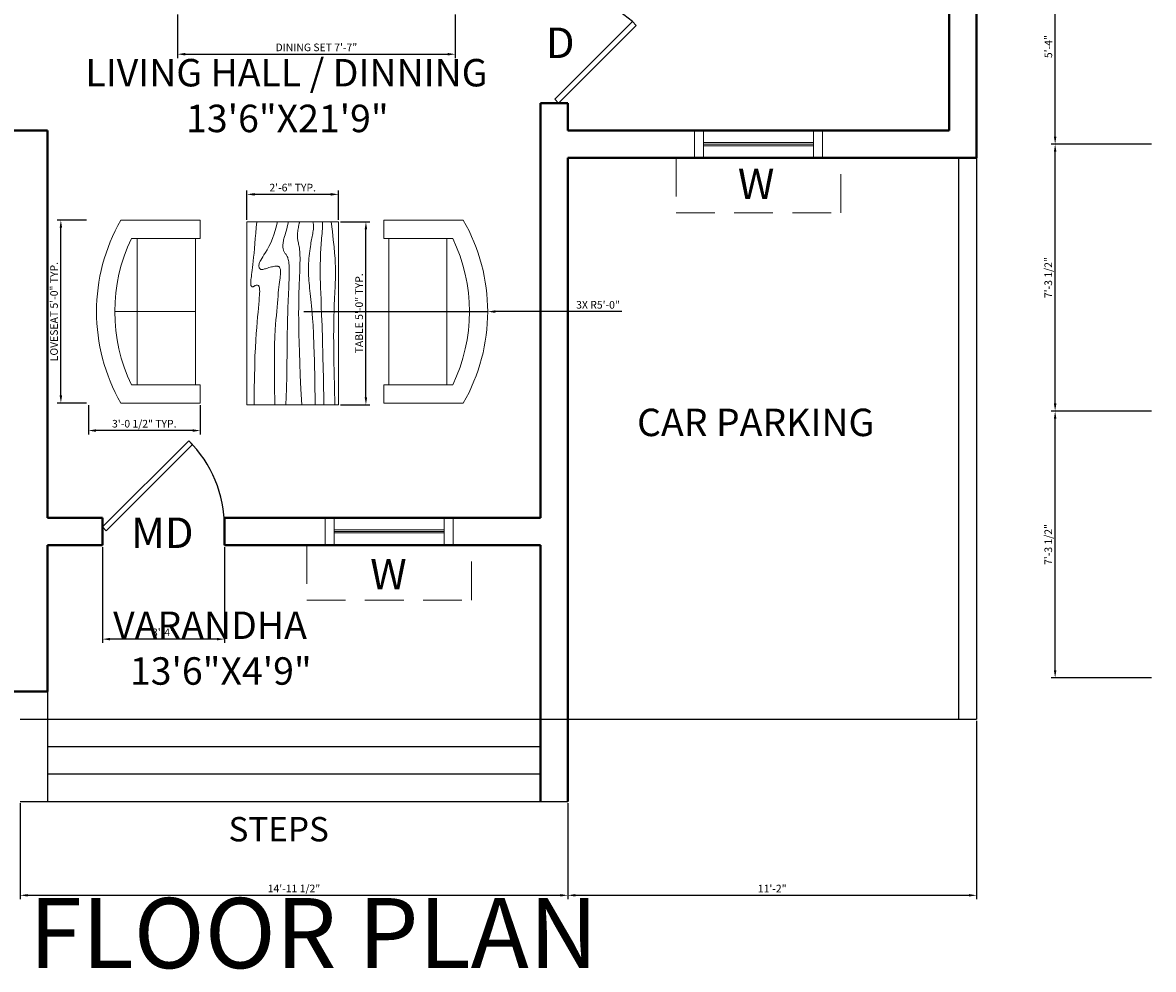
# Model space of a CAD drawing. Units: inches. Extents: x 4878 to 9282, y 5367 to 6617.
# Tile 5 of 14: x 5133 to 5503, y 5765 to 6075. Entities that reach past the tile are written whole.
import ezdxf

# ---------------------------------------------------------------- set-up
doc = ezdxf.new("R2010")
doc.units = ezdxf.units.IN
doc.linetypes.add('DASHED', pattern=[19.05, 12.7, -6.35])
for name, color, linetype, lineweight in [('A-ANNO-DIMS', 2, 'Continuous', 18), ('A-ANNO-TEXT', 7, 'Continuous', 18), ('A-ANNO-TITL', 3, 'Continuous', 30), ('A-AREA-IDEN', 4, 'Continuous', 18), ('A-DOOR', 3, 'Continuous', 25), ('A-FLOR-STRS', 7, 'Continuous', 25), ('A-FURN', 8, 'Continuous', 18), ('A-GLAZ', 30, 'Continuous', 20), ('A-ROOF-OVHD', 8, 'DASHED', 13), ('A-SITE', 7, 'Continuous', 25), ('A-WALL', 7, 'Continuous', 40)]:
    doc.layers.add(name, color=color, linetype=linetype, lineweight=lineweight)
doc.styles.get("Standard").update_dxf_attribs({"font": 'arial.ttf'})
doc.dimstyles.new('ISO-25', dxfattribs={"dimtxt": 2.5, "dimasz": 2.5, "dimexe": 1.25, "dimexo": 0.625, "dimtad": 1, "dimdec": 0, "dimlunit": 3, "dimtxsty": 'Standard', "dimcen": 2.5, "dimadec": 0, "dimazin": 0, "dimtfac": 1, "dimtdec": 0, "dimtmove": 0, "dimatfit": 3, "dimfxl": 1, "dimarcsym": 0})

# ---------------------------------------------------------------- blocks, each defined once
blk = doc.blocks.new('Sofa - Roundback Loveseat 5 ft.')
for p, q in [((0, -32.44198), (0, -5.99998)), ((-24, -33.99998), (-24, -11.46958)), ((-23.9998, -13.38178), (23.99986, -13.38178)), ((24.00004, -33.99998), (24.00004, -11.46958)), ((-24, -32.44198), (24.00004, -32.44198))]:
    blk.add_line(p, q)
for points in [[(-24, -33.99998), (-30, -33.99998), (-30, -7.99998)], [(30.00004, -7.99998), (30.00004, -33.99998), (24.00004, -33.99998)]]:
    blk.add_lwpolyline(points)
for centre, radius, start, end in [((0, -60.24998), 60.24998, 60.13715, 119.8628), ((0, -61.38438), 55.38444, 64.32083, 115.6792)]:
    blk.add_arc(centre, radius, start, end)
blk = doc.blocks.new('Table - Rectangular Woodgrain 60 x 30 in.')
for p, q in [((0, 0), (0, -30)), ((60, 0), (0, 0)), ((60, -30), (60, 0)), ((0, -30), (60, -30))]:
    blk.add_line(p, q)
for points in [[(0, -2.4), (4.8155, -2.418), (9.0302, -2.4688), (12.709, -2.5477), (15.9167, -2.65), (18.7181, -2.7711), (21.1781, -2.9063), (23.3616, -3.0508), (25.3333, -3.2), (27.1477, -3.3495), (28.8172, -3.4958), (30.3437, -3.636), (31.7291, -3.7667), (32.9756, -3.8849), (34.0849, -3.9875), (35.059, -4.0714), (35.9, -4.1334), (36.6114, -4.1711), (37.2041, -4.1854), (37.6906, -4.1779), (38.0833, -4.15), (38.3948, -4.1034), (38.6375, -4.0396), (38.8239, -3.9602), (38.9666, -3.8667), (39.0764, -3.7608), (39.1573, -3.6448), (39.2116, -3.521), (39.2416, -3.3917), (39.2498, -3.2593), (39.2385, -3.1261), (39.21, -2.9944), (39.1666, -2.8667), (39.111, -2.7447), (39.0468, -2.6281), (38.978, -2.5163), (38.9083, -2.4083), (38.8418, -2.3035), (38.7823, -2.201), (38.7337, -2.1001), (38.7, -2), (38.6844, -1.9003), (38.6875, -1.8021), (38.7094, -1.707), (38.75, -1.6167), (38.8094, -1.5326), (38.8875, -1.4563), (38.9844, -1.3893), (39.1, -1.3333), (39.2351, -1.2896), (39.3937, -1.2583), (39.5804, -1.2396), (39.8, -1.2333), (40.057, -1.2396), (40.3562, -1.2583), (40.7023, -1.2896), (41.1, -1.3333), (41.5547, -1.3895), (42.0755, -1.4573), (42.6721, -1.5361), (43.3542, -1.625), (44.1316, -1.7233), (45.014, -1.8302), (46.0114, -1.9449), (47.1333, -2.0667), (48.3862, -2.1947), (49.7625, -2.3281), (51.2513, -2.4663), (52.8416, -2.6083), (54.5226, -2.7535), (56.2833, -2.9011), (58.1127, -3.0501), (60, -3.2)], [(0, -9.2), (6.5759, -9.0858), (11.9385, -9.0365), (16.2527, -9.0418), (19.6833, -9.0917), (22.3952, -9.1759), (24.5531, -9.2844), (26.322, -9.4069), (27.8666, -9.5333), (29.3241, -9.6553), (30.7203, -9.7719), (32.0532, -9.8837), (33.3208, -9.9917), (34.5213, -10.0965), (35.6526, -10.199), (36.7128, -10.2999), (37.7, -10.4), (38.6129, -10.4996), (39.4531, -10.5969), (40.223, -10.6895), (40.925, -10.775), (41.5613, -10.8512), (42.1344, -10.9156), (42.6465, -10.966), (43.1, -11), (43.4976, -11.0158), (43.8437, -11.0136), (44.143, -10.9942), (44.4, -10.9583), (44.6195, -10.9069), (44.8062, -10.8406), (44.9648, -10.7603), (45.1, -10.6667), (45.2155, -10.5598), (45.3114, -10.4365), (45.3871, -10.2929), (45.4416, -10.125), (45.4743, -9.929), (45.4844, -9.7011), (45.4709, -9.4371), (45.4333, -9.1333), (45.3716, -8.7883), (45.2896, -8.4104), (45.1919, -8.0107), (45.0833, -7.6), (44.9685, -7.1893), (44.8521, -6.7896), (44.7388, -6.4117), (44.6333, -6.0667), (44.54, -5.7628), (44.4614, -5.4979), (44.4001, -5.2675), (44.3583, -5.0667), (44.3384, -4.8909), (44.3427, -4.7354), (44.3736, -4.5956), (44.4333, -4.4667), (44.5236, -4.3453), (44.6427, -4.2333), (44.7884, -4.1339), (44.9583, -4.05), (45.1501, -3.9849), (45.3614, -3.9417), (45.59, -3.9234), (45.8333, -3.9333), (46.0915, -3.9749), (46.3734, -4.0531), (46.6906, -4.1736), (47.0542, -4.3417), (47.4756, -4.5629), (47.9661, -4.8427), (48.5372, -5.1866), (49.2, -5.6), (49.9676, -6.0844), (50.8594, -6.625), (51.8965, -7.2031), (53.1, -7.8), (54.491, -8.3969), (56.0906, -8.975), (57.9199, -9.5156), (60, -10)], [(0, -12.8), (5.1847, -12.9322), (9.6213, -13.0323), (13.3963, -13.1059), (16.5958, -13.1583), (19.3063, -13.1952), (21.614, -13.2219), (23.6054, -13.2439), (25.3666, -13.2667), (26.9728, -13.2947), (28.4531, -13.3281), (29.8256, -13.3663), (31.1083, -13.4083), (32.3191, -13.4535), (33.476, -13.501), (34.597, -13.5501), (35.7, -13.6), (36.7984, -13.6497), (37.8875, -13.6979), (38.9578, -13.743), (40, -13.7833), (41.0047, -13.8174), (41.9625, -13.8438), (42.864, -13.8607), (43.7, -13.8667), (44.4631, -13.8604), (45.1552, -13.8417), (45.7801, -13.8104), (46.3416, -13.7667), (46.8439, -13.7104), (47.2906, -13.6417), (47.6858, -13.5604), (48.0333, -13.4667), (48.3375, -13.3608), (48.6042, -13.2448), (48.8396, -13.121), (49.05, -12.9917), (49.2417, -12.8593), (49.4208, -12.7261), (49.5937, -12.5944), (49.7667, -12.4667), (49.9452, -12.3451), (50.1323, -12.2313), (50.3303, -12.1268), (50.5416, -12.0333), (50.7686, -11.9524), (51.0135, -11.8854), (51.2788, -11.8341), (51.5666, -11.8), (51.8785, -11.7843), (52.2116, -11.7865), (52.562, -11.8059), (52.926, -11.8417), (53.2998, -11.8931), (53.6795, -11.9594), (54.0614, -12.0397), (54.4416, -12.1333), (54.8223, -12.2401), (55.2293, -12.3625), (55.6942, -12.5037), (56.2489, -12.6667), (56.9251, -12.8547), (57.7545, -13.0708), (58.7689, -13.3182), (60, -13.6)], [(0, -18), (5.124, -17.7273), (9.6609, -17.5057), (13.6705, -17.3303), (17.2125, -17.1958), (20.3467, -17.0973), (23.1328, -17.0297), (25.6307, -16.9878), (27.9, -16.9667), (29.9928, -16.9617), (31.9302, -16.9703), (33.7254, -16.9907), (35.3917, -17.0208), (36.9423, -17.0588), (38.3906, -17.1026), (39.7499, -17.1503), (41.0333, -17.2), (42.2519, -17.2496), (43.4073, -17.2969), (44.4986, -17.3395), (45.525, -17.375), (46.4858, -17.4012), (47.3802, -17.4156), (48.2074, -17.416), (48.9667, -17.4), (49.6583, -17.3662), (50.2872, -17.3167), (50.8595, -17.2547), (51.3812, -17.1833), (51.8584, -17.1057), (52.2971, -17.025), (52.7034, -16.9443), (53.0833, -16.8667), (53.443, -16.7951), (53.789, -16.7313), (54.128, -16.6768), (54.4666, -16.6334), (54.8115, -16.6024), (55.1693, -16.5854), (55.5465, -16.5841), (55.95, -16.6), (56.3828, -16.6337), (56.8346, -16.6823), (57.2915, -16.7418), (57.7396, -16.8084), (58.165, -16.878), (58.5539, -16.9469), (58.8924, -17.0111), (59.1666, -17.0667), (59.3679, -17.1107), (59.5078, -17.1438), (59.6032, -17.1675), (59.6708, -17.1833), (59.7275, -17.193), (59.7901, -17.1979), (59.8753, -17.1998), (60, -17.2)], [(0, -22.4), (8.0098, -22.2501), (14.4094, -22.1011), (19.4168, -21.9535), (23.25, -21.8083), (26.1269, -21.6663), (28.2656, -21.5281), (29.884, -21.3947), (31.2, -21.2667), (32.3967, -21.1448), (33.5172, -21.0292), (34.5697, -20.9198), (35.5625, -20.8167), (36.5037, -20.7198), (37.4015, -20.6292), (38.2642, -20.5448), (39.1, -20.4667), (39.9164, -20.3951), (40.7187, -20.3313), (41.5117, -20.2768), (42.3, -20.2333), (43.0883, -20.2024), (43.8812, -20.1854), (44.6836, -20.1841), (45.5, -20.2), (46.3328, -20.234), (47.1747, -20.2844), (48.0163, -20.3488), (48.8479, -20.425), (49.66, -20.5106), (50.4429, -20.6031), (51.1872, -20.7004), (51.8833, -20.8), (52.5246, -20.8999), (53.1166, -20.9995), (53.6681, -21.0983), (54.1875, -21.1958), (54.6834, -21.2919), (55.1646, -21.3859), (55.6394, -21.4777), (56.1167, -21.5667), (56.6028, -21.6515), (57.0961, -21.7266), (57.5929, -21.7852), (58.0896, -21.8208), (58.5823, -21.8268), (59.0674, -21.7964), (59.5412, -21.723), (60, -21.6)], [(0, -25.2), (8.6355, -25.0504), (15.7026, -24.9031), (21.4049, -24.7606), (25.9458, -24.625), (29.529, -24.4988), (32.3578, -24.3844), (34.6359, -24.284), (36.5667, -24.2), (38.3213, -24.1341), (39.9417, -24.0854), (41.437, -24.0523), (42.8167, -24.0333), (44.0901, -24.0268), (45.2667, -24.0313), (46.3557, -24.0451), (47.3667, -24.0667), (48.309, -24.0947), (49.1928, -24.1287), (50.0284, -24.168), (50.826, -24.2125), (51.5959, -24.2617), (52.3483, -24.3151), (53.0935, -24.3725), (53.8417, -24.4334), (54.6009, -24.497), (55.3699, -24.561), (56.1454, -24.6226), (56.9239, -24.6792), (57.7021, -24.7279), (58.4764, -24.7662), (59.2435, -24.7911), (60, -24.8)], [(0, -28.8), (5.6867, -28.6681), (10.45, -28.5698), (14.407, -28.5012), (17.675, -28.4584), (20.3711, -28.4374), (22.6125, -28.4344), (24.5164, -28.4455), (26.2, -28.4667), (27.762, -28.4947), (29.2276, -28.5281), (30.6033, -28.5663), (31.8958, -28.6084), (33.1118, -28.6535), (34.2578, -28.7011), (35.3405, -28.7501), (36.3666, -28.8), (37.3443, -28.8497), (38.288, -28.8974), (39.2137, -28.9412), (40.1375, -28.9792), (41.0753, -29.0093), (42.0432, -29.0297), (43.0572, -29.0384), (44.1333, -29.0333), (45.2936, -29.0114), (46.5843, -28.9641), (48.0579, -28.8816), (49.7666, -28.7542), (51.7629, -28.5721), (54.0989, -28.3255), (56.8272, -28.0048), (60, -27.6)]]:
    blk.add_lwpolyline(points)
blk = doc.blocks.new('*U9')
for p, q in [((0, 0), (0, -6)), ((40, 0), (40, -6))]:
    blk.add_line(p, q)
blk.add_lwpolyline([(0, 0), (28.28, 28.28), (29.52, 27.05), (1.24, -1.24)], close=True)
blk.add_arc((0, 0), 40, 0, 45)
blk = doc.blocks.new('*U13')
for p, q in [((0, 0), (0, -6)), ((-36, 0), (-36, -6))]:
    blk.add_line(p, q)
blk.add_lwpolyline([(0, 0), (-25.46, 25.46), (-26.69, 24.22), (-1.24, -1.24)], close=True)
blk.add_arc((0, 0), 36, 135, 180)
blk = doc.blocks.new('WINDOW-PLAN-36IN')
for p, q in [((0, 0), (0, 9)), ((3, 0), (3, 9)), ((39, 0), (39, 9)), ((42, 0), (42, 9)), ((3, 5), (39, 5)), ((3, 4.5), (39, 4.5)), ((3, 4), (39, 4))]:
    blk.add_line(p, q)
blk = doc.blocks.new('WINDOW-HOOD-54IN')
for p, q in [((0, 18), (0, 0)), ((54, 0), (54, 18)), ((0, 0), (54, 0))]:
    blk.add_line(p, q)
blk = doc.blocks.new('*D57')
at = {"layer": 'A-ANNO-DIMS', "color": 0, "lineweight": -2, "transparency": 16777216}
for p, q in [((5153.72, 6010.24), (5144.09, 6010.24)), ((5145.34, 5952.74), (5145.34, 6007.74)), ((5153.72, 5950.24), (5144.09, 5950.24))]:
    blk.add_line(p, q, dxfattribs=at)
at = {"layer": 'A-ANNO-DIMS', "color": 0, "transparency": 16777216}
for points in [[(5144.93, 6007.74), (5145.76, 6007.74), (5145.34, 6010.24)], [(5144.93, 5952.74), (5145.76, 5952.74), (5145.34, 5950.24)]]:
    blk.add_solid(points, dxfattribs=at)
at = {"layer": 'Defpoints', "color": 0, "transparency": 16777216}
for p in [(5145.34, 6010.24), (5154.34, 6010.24), (5154.34, 5950.24)]:
    blk.add_point(p, dxfattribs=at)
at = {"layer": 'A-ANNO-DIMS', "color": 0, "transparency": 16777216, "insert": (5143.42, 5980.24), "char_height": 2.5, "attachment_point": 5, "rotation": 90}
blk.add_mtext('LOVESEAT 5\'-0" TYP.', dxfattribs=at)
blk = doc.blocks.new('*D58')
at = {"layer": 'A-ANNO-DIMS', "color": 0, "lineweight": -2, "transparency": 16777216}
for p, q in [((5154.34, 5949.62), (5154.34, 5939.99)), ((5191.01, 5949.62), (5191.01, 5939.99)), ((5188.51, 5941.24), (5156.84, 5941.24))]:
    blk.add_line(p, q, dxfattribs=at)
at = {"layer": 'A-ANNO-DIMS', "color": 0, "transparency": 16777216}
for points in [[(5156.84, 5941.66), (5156.84, 5940.83), (5154.34, 5941.24)], [(5188.51, 5941.66), (5188.51, 5940.83), (5191.01, 5941.24)]]:
    blk.add_solid(points, dxfattribs=at)
at = {"layer": 'Defpoints', "color": 0, "transparency": 16777216}
for p in [(5154.34, 5950.24), (5191.01, 5950.24), (5154.34, 5941.24)]:
    blk.add_point(p, dxfattribs=at)
at = {"layer": 'A-ANNO-DIMS', "color": 0, "transparency": 16777216, "insert": (5172.68, 5943.16), "char_height": 2.5, "attachment_point": 5}
blk.add_mtext('3\'-0 1/2" TYP.', dxfattribs=at)
blk = doc.blocks.new('*D59')
at = {"layer": 'A-ANNO-DIMS', "color": 0, "lineweight": -2, "transparency": 16777216}
for p, q in [((5236.94, 6009.69), (5246.56, 6009.69)), ((5245.31, 5952.19), (5245.31, 6007.19)), ((5236.94, 5949.69), (5246.56, 5949.69))]:
    blk.add_line(p, q, dxfattribs=at)
at = {"layer": 'A-ANNO-DIMS', "color": 0, "transparency": 16777216}
for points in [[(5244.89, 6007.19), (5245.73, 6007.19), (5245.31, 6009.69)], [(5244.89, 5952.19), (5245.73, 5952.19), (5245.31, 5949.69)]]:
    blk.add_solid(points, dxfattribs=at)
at = {"layer": 'Defpoints', "color": 0, "transparency": 16777216}
for p in [(5236.31, 6009.69), (5245.31, 6009.69), (5236.31, 5949.69)]:
    blk.add_point(p, dxfattribs=at)
at = {"layer": 'A-ANNO-DIMS', "color": 0, "transparency": 16777216, "insert": (5243.41, 5979.69), "char_height": 2.5, "attachment_point": 5, "rotation": 90}
blk.add_mtext('TABLE 5\'-0" TYP.', dxfattribs=at)
blk = doc.blocks.new('*D60')
at = {"layer": 'A-ANNO-DIMS', "color": 0, "lineweight": -2, "transparency": 16777216}
for p, q in [((5206.31, 6010.32), (5206.31, 6019.94)), ((5233.81, 6018.69), (5208.81, 6018.69)), ((5236.31, 6010.32), (5236.31, 6019.94))]:
    blk.add_line(p, q, dxfattribs=at)
at = {"layer": 'A-ANNO-DIMS', "color": 0, "transparency": 16777216}
for points in [[(5208.81, 6019.11), (5208.81, 6018.27), (5206.31, 6018.69)], [(5233.81, 6019.11), (5233.81, 6018.27), (5236.31, 6018.69)]]:
    blk.add_solid(points, dxfattribs=at)
at = {"layer": 'Defpoints', "color": 0, "transparency": 16777216}
for p in [(5206.31, 6018.69), (5206.31, 6009.69), (5236.31, 6009.69)]:
    blk.add_point(p, dxfattribs=at)
at = {"layer": 'A-ANNO-DIMS', "color": 0, "transparency": 16777216, "insert": (5221.31, 6020.59), "char_height": 2.5, "attachment_point": 5}
blk.add_mtext('2\'-6" TYP.', dxfattribs=at)
blk = doc.blocks.new('*D61')
at = {"layer": 'A-ANNO-DIMS', "color": 0, "lineweight": -2, "transparency": 16777216}
for p, q in [((5183.58, 6077.68), (5183.58, 6063.4)), ((5274.58, 6077.68), (5274.58, 6063.4)), ((5186.08, 6064.65), (5272.08, 6064.65))]:
    blk.add_line(p, q, dxfattribs=at)
at = {"layer": 'A-ANNO-DIMS', "color": 0, "transparency": 16777216}
for points in [[(5186.08, 6065.07), (5186.08, 6064.23), (5183.58, 6064.65)], [(5272.08, 6065.07), (5272.08, 6064.23), (5274.58, 6064.65)]]:
    blk.add_solid(points, dxfattribs=at)
at = {"layer": 'Defpoints', "color": 0, "transparency": 16777216}
for p in [(5183.58, 6078.3), (5274.58, 6078.3), (5274.58, 6064.65)]:
    blk.add_point(p, dxfattribs=at)
at = {"layer": 'A-ANNO-DIMS', "color": 0, "transparency": 16777216, "insert": (5229.08, 6066.57), "char_height": 2.5, "attachment_point": 5}
blk.add_mtext('DINING SET 7\'-7"', dxfattribs=at)
blk = doc.blocks.new('*D72')
at = {"layer": 'A-ANNO-DIMS', "color": 0, "lineweight": -2, "transparency": 16777216}
for p, q in [((5502.78, 5947.64), (5469.95, 5947.64)), ((5471.2, 5862.64), (5471.2, 5945.14)), ((5502.78, 5860.14), (5469.95, 5860.14))]:
    blk.add_line(p, q, dxfattribs=at)
at = {"layer": 'A-ANNO-DIMS', "color": 0, "transparency": 16777216}
for points in [[(5470.79, 5945.14), (5471.62, 5945.14), (5471.2, 5947.64)], [(5470.79, 5862.64), (5471.62, 5862.64), (5471.2, 5860.14)]]:
    blk.add_solid(points, dxfattribs=at)
at = {"layer": 'Defpoints', "color": 0, "transparency": 16777216}
for p in [(5471.2, 5947.64), (5503.4, 5947.64), (5503.4, 5860.14)]:
    blk.add_point(p, dxfattribs=at)
at = {"layer": 'A-ANNO-DIMS', "color": 0, "transparency": 16777216, "insert": (5469.28, 5903.89), "char_height": 2.5, "attachment_point": 5, "rotation": 90}
blk.add_mtext('7\'-3 1/2"', dxfattribs=at)
blk = doc.blocks.new('*D73')
at = {"layer": 'A-ANNO-DIMS', "color": 0, "lineweight": -2, "transparency": 16777216}
for p, q in [((5502.78, 6035.14), (5469.95, 6035.14)), ((5471.2, 5950.14), (5471.2, 6032.64)), ((5502.78, 5947.64), (5469.95, 5947.64))]:
    blk.add_line(p, q, dxfattribs=at)
at = {"layer": 'A-ANNO-DIMS', "color": 0, "transparency": 16777216}
for points in [[(5470.79, 6032.64), (5471.62, 6032.64), (5471.2, 6035.14)], [(5470.79, 5950.14), (5471.62, 5950.14), (5471.2, 5947.64)]]:
    blk.add_solid(points, dxfattribs=at)
at = {"layer": 'Defpoints', "color": 0, "transparency": 16777216}
for p in [(5471.2, 6035.14), (5503.4, 6035.14), (5503.4, 5947.64)]:
    blk.add_point(p, dxfattribs=at)
at = {"layer": 'A-ANNO-DIMS', "color": 0, "transparency": 16777216, "insert": (5469.28, 5991.39), "char_height": 2.5, "attachment_point": 5, "rotation": 90}
blk.add_mtext('7\'-3 1/2"', dxfattribs=at)
blk = doc.blocks.new('*D74')
at = {"layer": 'A-ANNO-DIMS', "color": 0, "lineweight": -2, "transparency": 16777216}
for p, q in [((5502.78, 6099.14), (5469.95, 6099.14)), ((5471.2, 6037.64), (5471.2, 6096.64)), ((5502.78, 6035.14), (5469.95, 6035.14))]:
    blk.add_line(p, q, dxfattribs=at)
at = {"layer": 'A-ANNO-DIMS', "color": 0, "transparency": 16777216}
for points in [[(5470.79, 6096.64), (5471.62, 6096.64), (5471.2, 6099.14)], [(5470.79, 6037.64), (5471.62, 6037.64), (5471.2, 6035.14)]]:
    blk.add_solid(points, dxfattribs=at)
at = {"layer": 'Defpoints', "color": 0, "transparency": 16777216}
for p in [(5471.2, 6099.14), (5503.4, 6099.14), (5503.4, 6035.14)]:
    blk.add_point(p, dxfattribs=at)
at = {"layer": 'A-ANNO-DIMS', "color": 0, "transparency": 16777216, "insert": (5469.31, 6067.14), "char_height": 2.5, "attachment_point": 5, "rotation": 90}
blk.add_mtext('5\'-4"', dxfattribs=at)
blk = doc.blocks.new('*D102')
at = {"layer": 'A-ANNO-DIMS', "color": 0, "lineweight": -2, "transparency": 16777216}
for p, q in [((5131.98, 5819.02), (5131.98, 5787.59)), ((5311.48, 5819.02), (5311.48, 5787.59)), ((5134.48, 5788.84), (5308.98, 5788.84))]:
    blk.add_line(p, q, dxfattribs=at)
at = {"layer": 'A-ANNO-DIMS', "color": 0, "transparency": 16777216}
for points in [[(5134.48, 5789.26), (5134.48, 5788.43), (5131.98, 5788.84)], [(5308.98, 5789.26), (5308.98, 5788.43), (5311.48, 5788.84)]]:
    blk.add_solid(points, dxfattribs=at)
at = {"layer": 'Defpoints', "color": 0, "transparency": 16777216}
for p in [(5131.98, 5819.64), (5311.48, 5819.64), (5311.48, 5788.84)]:
    blk.add_point(p, dxfattribs=at)
at = {"layer": 'A-ANNO-DIMS', "color": 0, "transparency": 16777216, "insert": (5221.73, 5790.76), "char_height": 2.5, "attachment_point": 5}
blk.add_mtext('14\'-11 1/2"', dxfattribs=at)
blk = doc.blocks.new('*D103')
at = {"layer": 'A-ANNO-DIMS', "color": 0, "lineweight": -2, "transparency": 16777216}
for p, q in [((5445.48, 5846.02), (5445.48, 5787.59)), ((5311.48, 5819.02), (5311.48, 5787.59)), ((5313.98, 5788.84), (5442.98, 5788.84))]:
    blk.add_line(p, q, dxfattribs=at)
at = {"layer": 'A-ANNO-DIMS', "color": 0, "transparency": 16777216}
for points in [[(5313.98, 5789.26), (5313.98, 5788.43), (5311.48, 5788.84)], [(5442.98, 5789.26), (5442.98, 5788.43), (5445.48, 5788.84)]]:
    blk.add_solid(points, dxfattribs=at)
at = {"layer": 'Defpoints', "color": 0, "transparency": 16777216}
for p in [(5445.48, 5846.64), (5311.48, 5819.64), (5445.48, 5788.84)]:
    blk.add_point(p, dxfattribs=at)
at = {"layer": 'A-ANNO-DIMS', "color": 0, "transparency": 16777216, "insert": (5378.48, 5790.72), "char_height": 2.5, "attachment_point": 5}
blk.add_mtext('11\'-2"', dxfattribs=at)
blk = doc.blocks.new('*D104')
at = {"layer": 'A-ANNO-DIMS', "color": 0, "lineweight": -2, "transparency": 16777216}
for p, q in [((5158.98, 5903.02), (5158.98, 5871.59)), ((5198.98, 5903.02), (5198.98, 5871.59)), ((5196.48, 5872.84), (5161.48, 5872.84))]:
    blk.add_line(p, q, dxfattribs=at)
at = {"layer": 'A-ANNO-DIMS', "color": 0, "transparency": 16777216}
for points in [[(5161.48, 5873.26), (5161.48, 5872.43), (5158.98, 5872.84)], [(5196.48, 5873.26), (5196.48, 5872.43), (5198.98, 5872.84)]]:
    blk.add_solid(points, dxfattribs=at)
at = {"layer": 'Defpoints', "color": 0, "transparency": 16777216}
for p in [(5158.98, 5903.64), (5198.98, 5903.64), (5158.98, 5872.84)]:
    blk.add_point(p, dxfattribs=at)
at = {"layer": 'A-ANNO-DIMS', "color": 0, "transparency": 16777216, "insert": (5178.98, 5874.75), "char_height": 2.5, "attachment_point": 5}
blk.add_mtext('3\'-4"', dxfattribs=at)
blk = doc.blocks.new('*D122')
at = {"layer": 'A-ANNO-DIMS', "color": 0, "lineweight": -2, "transparency": 16777216}
for p, q in [((5224.98, 5980.24), (5285.23, 5980.24)), ((5329.2, 5980.24), (5287.73, 5980.24))]:
    blk.add_line(p, q, dxfattribs=at)
at = {"layer": 'A-ANNO-DIMS', "color": 0, "transparency": 16777216}
blk.add_solid([(5287.73, 5980.66), (5287.73, 5979.83), (5285.23, 5980.24)], dxfattribs=at)
at = {"layer": 'Defpoints', "color": 0, "transparency": 16777216}
for p in [(5224.98, 5980.24), (5285.23, 5980.24)]:
    blk.add_point(p, dxfattribs=at)
at = {"layer": 'A-ANNO-DIMS', "color": 0, "transparency": 16777216, "insert": (5321.38, 5982.15), "char_height": 2.5, "attachment_point": 5, "rotation": 0.0001}
blk.add_mtext('3X R5\'-0"', dxfattribs=at)

msp = doc.modelspace()

# ---------------------------------------------------------------- linework, layer by layer
at = {"layer": 'A-FLOR-STRS'}
for p, q in [((5140.98, 5855.64), (5140.98, 5819.64)), ((5131.98, 5846.64), (5311.48, 5846.64)), ((5140.98, 5837.64), (5302.48, 5837.64)), ((5140.98, 5828.64), (5302.48, 5828.64)), ((5131.98, 5819.64), (5311.48, 5819.64))]:
    msp.add_line(p, q, dxfattribs=at)
at = {"layer": 'A-SITE'}
for p, q in [((5439.48, 6030.64), (5439.48, 5846.64)), ((5445.48, 6030.64), (5445.48, 5846.64)), ((5311.48, 5846.64), (5445.48, 5846.64))]:
    msp.add_line(p, q, dxfattribs=at)
at = {"layer": 'A-WALL'}
for p, q in [((5445.48, 6182.64), (5445.48, 6030.64)), ((5436.48, 6173.64), (5436.48, 6039.64)), ((5311.48, 6048.64), (5302.48, 6048.64)), ((5302.48, 6048.64), (5302.48, 6039.64)), ((5311.48, 6048.64), (5311.48, 6039.64)), ((5140.98, 6039.64), (5125.98, 6039.64)), ((5140.98, 5912.64), (5140.98, 6039.64)), ((5302.48, 5912.64), (5302.48, 6039.64)), ((5436.48, 6039.64), (5311.48, 6039.64)), ((5445.48, 6030.64), (5311.48, 6030.64)), ((5311.48, 5819.64), (5311.48, 6030.64)), ((5158.98, 5912.64), (5140.98, 5912.64)), ((5158.98, 5903.64), (5158.98, 5912.64)), ((5203.43, 5912.64), (5198.98, 5912.64)), ((5198.98, 5903.64), (5198.98, 5912.64)), ((5302.48, 5912.64), (5203.43, 5912.64)), ((5140.98, 5855.64), (5140.98, 5903.64)), ((5158.98, 5903.64), (5140.98, 5903.64)), ((5203.43, 5903.64), (5198.98, 5903.64)), ((5302.48, 5903.64), (5203.43, 5903.64)), ((5302.48, 5819.64), (5302.48, 5903.64)), ((5140.98, 5855.64), (4988.98, 5855.64))]:
    msp.add_line(p, q, dxfattribs=at)

# ---------------------------------------------------------------- block references
at = {"layer": 'A-DOOR', "rotation": 270}
msp.add_blockref('*U13', (5308.48, 6048.64), dxfattribs=at)
at = {"layer": 'A-DOOR'}
msp.add_blockref('*U9', (5158.98, 5909.64), dxfattribs=at)
at = {"layer": 'A-FURN'}
for name, p, rotation in [('Sofa - Roundback Loveseat 5 ft.', (5157.01, 5980.24), 90), ('Table - Rectangular Woodgrain 60 x 30 in.', (5206.31, 5949.69), 90), ('Sofa - Roundback Loveseat 5 ft.', (5285.23, 5980.24), 270)]:
    msp.add_blockref(name, p, dxfattribs=dict(at, rotation=rotation))
at = {"layer": 'A-GLAZ'}
for p in [(5352.98, 6030.65), (5231.95, 5903.65)]:
    msp.add_blockref('WINDOW-PLAN-36IN', p, dxfattribs=at)
at = {"layer": 'A-ROOF-OVHD'}
for p in [(5346.98, 6012.65), (5225.95, 5885.64)]:
    msp.add_blockref('WINDOW-HOOD-54IN', p, dxfattribs=at)

# ---------------------------------------------------------------- texts
at = {"layer": 'A-ANNO-TEXT', "char_height": 10, "width": 649.8744, "attachment_point": 1}
for s, insert in [('D', (5304.32, 6073.39)), ('W', (5367.22, 6027.14)), ('MD', (5168.35, 5912.73)), ('W', (5246.71, 5899.17))]:
    msp.add_mtext(s, dxfattribs=dict(at, insert=insert))
at = {"layer": 'A-ANNO-TEXT', "insert": (5200.29, 5814.52), "char_height": 8, "attachment_point": 1}
msp.add_mtext_dynamic_manual_height_columns('STEPS', width=123.3151, gutter_width=12.5, heights=[0], dxfattribs=at)
at = {"layer": 'A-ANNO-TITL', "insert": (5134.86, 5787.96), "char_height": 23, "attachment_point": 1}
msp.add_mtext_dynamic_manual_height_columns('FLOOR PLAN', width=873.405, gutter_width=12.5, heights=[0], dxfattribs=at)
at = {"layer": 'A-AREA-IDEN', "char_height": 9, "attachment_point": 1}
for s, width, insert in [('LIVING HALL / DINNING\\P            13\'6"X21\'9"', 412.5838, (5153.37, 6063.09)), ('CAR PARKING ', 416.4936, (5334.19, 5948.42)), ('VARANDHA\\P  13\'6"X4\'9"', 524.8947, (5162.47, 5881.9))]:
    msp.add_mtext_dynamic_manual_height_columns(s, width=width, gutter_width=12.5, heights=[0], dxfattribs=dict(at, insert=insert))

# ---------------------------------------------------------------- dimensions: what is measured, and where the dimension line sits
at = {"layer": 'A-ANNO-DIMS'}
for base, p1, p2, angle, picture, middle in [((5471.2, 6099.14), (5503.4, 6035.14), (5503.4, 6099.14), 90, '*D74', (5469.31, 6067.14)), ((5471.2, 6035.14), (5503.4, 5947.64), (5503.4, 6035.14), 90, '*D73', (5469.28, 5991.39)), ((5471.2, 5947.64), (5503.4, 5860.14), (5503.4, 5947.64), 90, '*D72', (5469.28, 5903.89)), ((5158.98, 5872.84), (5198.98, 5903.64), (5158.98, 5903.64), 180, '*D104', (5178.98, 5874.75))]:
    dim = msp.add_linear_dim(base=base, p1=p1, p2=p2, angle=angle, dimstyle='ISO-25', override={"dimdec": 1, "dimlfac": 1, "dimrnd": 0, "dimzin": 1, "dimdsep": 46, "dimlunit": 4, "dimfrac": 2}, dxfattribs=at)
    dim.commit()
    dim.dimension.update_dxf_attribs({"geometry": picture, "text_midpoint": middle})
dim = msp.add_linear_dim(base=(5274.58, 6064.65), p1=(5183.58, 6078.3), p2=(5274.58, 6078.3), text='DINING SET <>', dimstyle='ISO-25', override={"dimdec": 1, "dimlfac": 1, "dimrnd": 0, "dimzin": 1, "dimdsep": 46, "dimlunit": 4, "dimfrac": 2}, dxfattribs=at)
dim.commit()
dim.dimension.update_dxf_attribs({"geometry": '*D61', "text_midpoint": (5229.08, 6066.57)})
for base, p1, p2, angle, text, picture, middle in [((5206.31, 6018.69), (5236.31, 6009.69), (5206.31, 6009.69), 180, '<> TYP.', '*D60', (5221.31, 6020.59)), ((5145.34, 6010.24), (5154.34, 5950.24), (5154.34, 6010.24), 90, 'LOVESEAT <> TYP.', '*D57', (5143.42, 5980.24)), ((5245.31, 6009.69), (5236.31, 5949.69), (5236.31, 6009.69), 90, 'TABLE <> TYP.', '*D59', (5243.41, 5979.69)), ((5154.34, 5941.24), (5191.01, 5950.24), (5154.34, 5950.24), 180, '<> TYP.', '*D58', (5172.68, 5943.16))]:
    dim = msp.add_linear_dim(base=base, p1=p1, p2=p2, angle=angle, text=text, dimstyle='ISO-25', override={"dimdec": 1, "dimlfac": 1, "dimrnd": 0, "dimzin": 1, "dimdsep": 46, "dimlunit": 4, "dimfrac": 2}, dxfattribs=at)
    dim.commit()
    dim.dimension.update_dxf_attribs({"geometry": picture, "text_midpoint": middle})
dim = msp.add_radius_dim(center=(5224.97523, 5980.24486), mpoint=(5285.22521, 5980.245), text='3X <>', dimstyle='ISO-25', override={"dimdec": 1, "dimlfac": 1, "dimrnd": 0, "dimzin": 1, "dimdsep": 46, "dimlunit": 4, "dimfrac": 2}, dxfattribs=at)
dim.commit()
dim.dimension.update_dxf_attribs({"geometry": '*D122', "text_midpoint": (5321.37519, 5980.24508), "dimtype": 164})
for base, p1, p2, picture, middle in [((5445.48, 5788.84), (5311.48, 5819.64), (5445.48, 5846.64), '*D103', (5378.48, 5790.72)), ((5311.48, 5788.84), (5131.98, 5819.64), (5311.48, 5819.64), '*D102', (5221.73, 5790.76))]:
    dim = msp.add_linear_dim(base=base, p1=p1, p2=p2, dimstyle='ISO-25', override={"dimdec": 1, "dimlfac": 1, "dimrnd": 0, "dimzin": 1, "dimdsep": 46, "dimlunit": 4, "dimfrac": 2}, dxfattribs=at)
    dim.commit()
    dim.dimension.update_dxf_attribs({"geometry": picture, "text_midpoint": middle})

doc.saveas('drawing.dxf')
